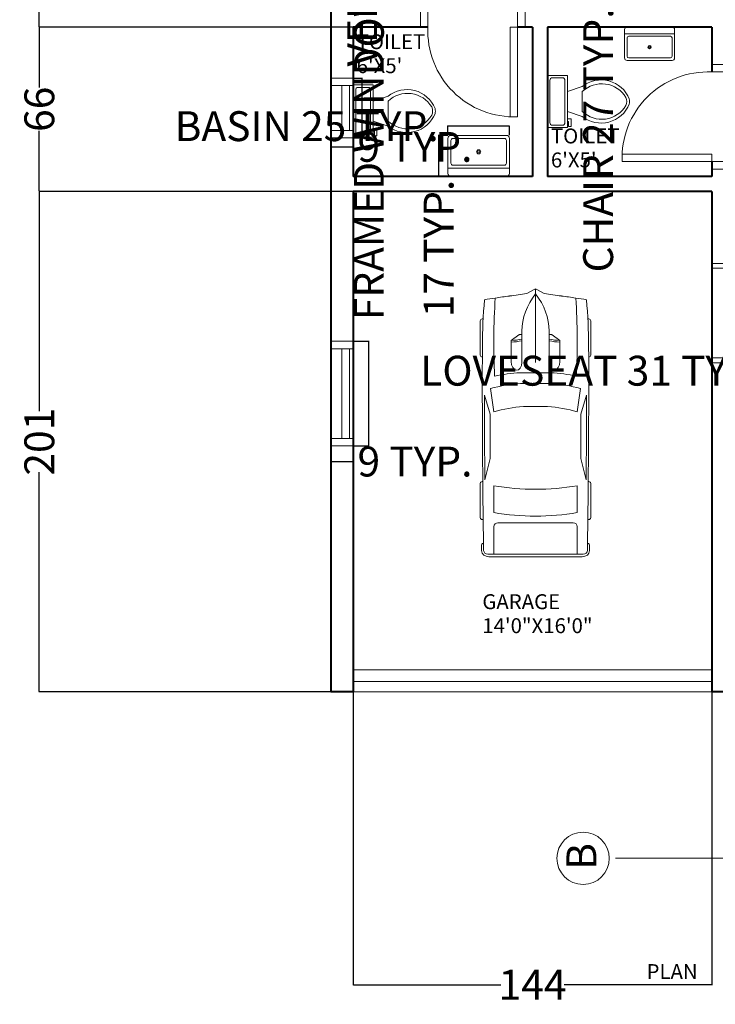
# Model space of a CAD drawing. Units: inches. Extents: x -101 to 786, y 26 to 880.
# Tile 1 of 9: x -101 to 178, y 26 to 422. Entities that reach past the tile are written whole.
import ezdxf

# ---------------------------------------------------------------- set-up
doc = ezdxf.new("R2010")
doc.units = ezdxf.units.IN
doc.header["$MEASUREMENT"] = 0
for name, color, linetype, lineweight in [('A-ANNO-DIMS', 2, 'Continuous', 18), ('A-ANNO-SYMB', 2, 'Continuous', 18), ('A-ANNO-TEXT', 7, 'Continuous', 25), ('A-AREA-IDEN', 7, 'Continuous', 18), ('A-DOOR', 4, 'Continuous', 20), ('A-EQPM-VEHC', 9, 'Continuous', 13), ('A-FLOR-FIXT', 8, 'Continuous', 18), ('A-GLAZ', 4, 'Continuous', 18), ('A-WALL', 7, 'Continuous', 40)]:
    doc.layers.add(name, color=color, linetype=linetype, lineweight=lineweight)
doc.styles.get("Standard").update_dxf_attribs({"font": 'arial.ttf'})
doc.dimstyles.get("Standard").update_dxf_attribs({"dimtxt": 12, "dimasz": 0.18, "dimexe": 0.18, "dimexo": 0.0625, "dimgap": 0.09, "dimtad": 0, "dimdec": 1, "dimzin": 0, "dimdsep": 46, "dimlunit": 3, "dimtxsty": 'Standard', "dimcen": 0.09, "dimadec": 0, "dimazin": 0, "dimtfac": 1, "dimtdec": 1, "dimtofl": 0, "dimtmove": 0, "dimatfit": 3, "dimfxl": 1, "dimtolj": 1, "dimtzin": 0, "dimarcsym": 0})

# ---------------------------------------------------------------- blocks, each defined once
blk = doc.blocks.new('Sink-single - 30 in top')
blk.add_line((-15, -3.999996), (15, -3.999996))
for points in [[(-13.5, 0), (13.5, 0)], [(-15, -18.499996), (-15, -1.5)], [(15, -1.5), (15, -18.499996)], [(-13.5, -17.499996), (-13.5, -6.499996)], [(-12.5, -5.499996), (12.5, -5.499996)], [(13.5, -6.499996), (13.5, -17.499996)], [(12.5, -18.499996), (-12.5, -18.499996)], [(13.5, -19.999996), (-13.5, -19.999996)]]:
    blk.add_lwpolyline(points)
for radius in [1, 0.5]:
    blk.add_circle((0, -11.999996), radius)
for centre, radius, start, end in [((-13.5, -1.5), 1.5, 90, 180), ((13.5, -1.5), 1.5, 0, 90), ((-12.5, -6.499996), 1, 90, 180), ((12.5, -6.499996), 1, 0, 90), ((-13.5, -18.499996), 1.5, 180, 270), ((-12.5, -17.499996), 1, 180, 270), ((12.5, -17.499996), 1, 270, 0), ((13.5, -18.499996), 1.5, 270, 0)]:
    blk.add_arc(centre, radius, start, end)
blk = doc.blocks.new('Toilet - top')
for p, q in [((9.5, -6), (9.5, -2)), ((-10, -8.5), (-8, -8.5)), ((-10, -9.5), (-10, -8.5)), ((-7, -9.5), (-10, -9.5)), ((-8, -8.5), (-8, -8)), ((-7, -8), (-7, -9.5)), ((-4, -8), (-6, -14)), ((4, -8), (6, -14)), ((4, -14), (-4, -14))]:
    blk.add_line(p, q)
blk.add_lwpolyline([(10.5, -8), (10.5, 0), (-10.5, 0), (-10.5, -8)], close=True)
for points in [[(-9.5, -2), (-9.5, -6)], [(8.5, -1), (-8.5, -1)], [(-8.5, -7), (8.5, -7)]]:
    blk.add_lwpolyline(points)
for centre, radius, start, end in [((-8.62, -1.88), 0.884, 81.8699, 188.1301), ((8.62, -1.88), 0.884, 351.8699, 98.1301), ((-8.62, -6.12), 0.884, 171.8699, 278.1301), ((8.62, -6.12), 0.884, 261.8699, 8.1301), ((3.52, -21.58), 12.17, 141.4691, 247.9714), ((4.2, -21.82), 11.33, 136.3677, 238.9468), ((-3.52, -21.58), 12.17, 292.0284, 38.5307), ((-4.2, -21.82), 11.33, 301.053, 43.6321), ((0, -27.88), 4, 245.7318, 294.2682), ((0, -29), 4, 254.8605, 285.1395)]:
    blk.add_arc(centre, radius, start, end)
blk = doc.blocks.new('*U14')
for p, q in [((21.1, 37.41), (21.1, 36.83)), ((46.55, 38.89), (22.35, 38.89)), ((47.8, 37.39), (47.8, 37.41)), ((87.99, 31.87), (74.76, 35.92)), ((134.31, 35.6), (119.29, 31.78)), ((135.45, 37.07), (135.45, 37.41)), ((136.7, 38.89), (160.9, 38.89)), ((162.15, 37.41), (162.15, 36.77)), ((70.03, 31.54), (86.41, 29.35)), ((138.42, 29.35), (157.25, 29.35)), ((186.47, 29.35), (167.01, 29.35)), ((186.47, -33.5), (186.47, 33.5)), ((188.4, -32.76), (188.4, 32.76)), ((164.52, 26.39), (164.52, -26.39)), ((32.27, 11.63), (36.13, 17.17)), ((36.13, 17.17), (50.94, 17.17)), ((29.77, 9.51), (51.68, 9.51)), ((32.12, 9.51), (32.12, 11.15)), ((58.92, -10.77), (58.92, 10.77)), ((66.55, -10.53), (66.55, 10.53)), ((82.74, 8.5), (82.74, -8.5)), ((186.47, -10.53), (186.47, 10.53)), ((3.27, 6.13), (0.1, 0.41)), ((0, 0), (51.68, 0)), ((0.1, -0.41), (3.27, -6.13)), ((29.77, -9.51), (51.68, -9.51)), ((32.12, -9.51), (32.12, -11.15)), ((32.27, -11.63), (36.13, -17.17)), ((36.13, -17.17), (50.94, -17.17)), ((86.41, -29.35), (70.03, -31.54)), ((87.99, -31.87), (74.76, -35.92)), ((134.31, -35.6), (119.29, -31.78)), ((157.25, -29.35), (138.42, -29.35)), ((167.01, -29.35), (186.47, -29.35)), ((21.1, -37.41), (21.1, -36.83)), ((46.55, -38.89), (22.35, -38.89)), ((47.8, -37.39), (47.8, -37.41)), ((135.45, -37.07), (135.45, -37.41)), ((136.7, -38.89), (160.9, -38.89)), ((162.15, -37.41), (162.15, -36.77))]:
    blk.add_line(p, q)
for centre, major_axis, ratio, start_param, end_param in [((266.03, -27.52), (0, 313.31), 0.842304, 1.367076, 1.39176), ((41.19, -490.86), (0, 528.23), 0.842304, 0.00281, 0.075598), ((22.35, 37.41), (0, -1.48), 0.842304, 3.141593, 4.712389), ((64.48, -10555.62), (0, 10593.03), 0.842304, -0.013397, 0.002797), ((46.55, 37.41), (0, 1.48), 0.842304, -1.570796, 0), ((64.48, -10555.62), (0, -10591.55), 0.842304, 3.133765, 3.140441), ((136.7, 37.41), (0, -1.48), 0.842304, 3.141593, 4.712389), ((160.9, 37.41), (0, 1.48), 0.842304, -1.570796, 0), ((180.63, 35.84), (0, 2.22), 0.842304, -0.013017, 1.249894), ((64.48, -10556.36), (0, 10595.31), 0.842304, -0.013397, -0.013017), ((183.98, 33.5), (0, -2.96), 0.842304, 1.570796, 3.128196), ((183.98, 32.76), (0, -5.25), 0.842304, 1.570796, 3.128196), ((259.18, -27.52), (0, -305.3), 0.842304, 4.528606, 4.561838), ((37.47, -593.96), (0, -623.33), 0.842304, 3.096046, 3.200911), ((134.4, 5.39), (0, -89.78), 0.842304, 4.449482, 4.652344), ((135.29, 5.39), (0, 81.77), 0.842304, 1.245306, 1.50788), ((149.6, 2.8), (0, -79.58), 0.842304, 4.372215, 4.640744), ((95.79, -3666.35), (0, -3698.24), 0.842304, 3.134049, 3.144098), ((17.08, 0), (0, 147.02), 0.842304, 4.511394, 4.913384), ((35.91, 0), (0, 147.02), 0.842304, 4.511394, 4.913384), ((167.01, 26.39), (0, 2.96), 0.842304, 0, 1.570796), ((-204.49, 52.4), (0, -250.96), 0.842304, 1.385369, 1.434372), ((13.04, 17.01), (0, 27.42), 0.842304, 4.435146, 4.718221), ((14.2, 17.01), (0, 27.42), 0.842304, 4.435146, 4.718221), ((50.79, 13.34), (6.34, -0.36), 0.603834, -1.395552, 1.581315), ((29.77, -46.66), (0, 56.17), 0.842304, 0, 0.590319), ((32.75, 11.15), (0, 0.74), 0.842304, 0.879714, 1.570796), ((0.62, 0), (0, -0.74), 0.842304, 4.131459, 5.293319), ((-204.49, -52.4), (0, 250.96), 0.842304, -1.434372, -1.385369), ((29.77, 46.66), (0, 56.17), 0.842304, 2.551274, 3.141593), ((32.75, -11.15), (0, -0.74), 0.842304, 4.712389, 5.403472), ((13.04, -17.01), (0, -27.42), 0.842304, 1.564964, 1.848039), ((14.2, -17.01), (0, -27.42), 0.842304, 1.564964, 1.848039), ((134.4, -5.39), (0, -89.78), 0.842304, -1.510751, -1.307889), ((135.29, -5.39), (0, -81.77), 0.842304, -1.50788, -1.245306), ((149.6, -2.8), (0, -79.58), 0.842304, -1.499151, -1.230623), ((259.18, 27.52), (0, 305.3), 0.842304, 1.721348, 1.754579), ((167.01, -26.39), (0, -2.96), 0.842304, 4.712389, 6.283185), ((266.03, 27.52), (0, 313.31), 0.842304, 1.749832, 1.774517), ((37.47, 593.96), (0, -623.33), 0.842304, -0.059319, 0.045547), ((95.79, 3666.35), (0, -3698.24), 0.842304, -0.002505, 0.007544), ((183.98, -33.5), (0, 2.96), 0.842304, 3.15499, 4.712389), ((183.98, -32.76), (0, -5.25), 0.842304, 0.013397, 1.570796), ((41.19, 490.86), (0, -528.23), 0.842304, -0.075598, -0.00281), ((22.35, -37.41), (0, 1.48), 0.842304, 1.570796, 3.141593), ((64.48, 10555.62), (0, 10593.03), 0.842304, 3.138796, 3.15499), ((46.55, -37.41), (0, -1.48), 0.842304, 0, 1.570796), ((64.48, 10555.62), (0, -10591.55), 0.842304, 0.001152, 0.007828), ((136.7, -37.41), (0, -1.48), 0.842304, -1.570796, 0), ((160.9, -37.41), (0, 1.48), 0.842304, 3.141593, 4.712389), ((180.63, -35.84), (0, -2.22), 0.842304, -1.249894, 0.013017), ((64.48, 10556.36), (0, 10595.31), 0.842304, 3.15461, 3.15499)]:
    blk.add_ellipse(centre, major_axis=major_axis, ratio=ratio, start_param=start_param, end_param=end_param)
at = {"extrusion": (0, 0, -1)}
blk.add_ellipse((50.79, -13.34), major_axis=(6.34, 0.36), ratio=0.603834, start_param=-1.395552, end_param=1.581315, dxfattribs=at)
blk = doc.blocks.new('DOOR-SINGLE-36')
for p, q in [((-39, 0), (-39, -6)), ((-36, 0), (-36, -6)), ((0, 0), (0, -6)), ((3, 0), (3, -6))]:
    blk.add_line(p, q)
blk.add_lwpolyline([(0, 0), (-3, 0), (-3, 36), (0, 36)], close=True)
blk.add_arc((-1.5, 1.5), 34.53, 87.5104, 182.4896)
blk = doc.blocks.new('WIN-36-WALL9-FRAMED')
for p, q in [((0, 42), (9, 42)), ((0, 3), (0, 39)), ((0, 39), (9, 39)), ((4.5, 3), (4.5, 39)), ((7.5, 3), (7.5, 39)), ((9, 39), (9, 3)), ((9, 3), (0, 3)), ((9, 0), (0, 0))]:
    blk.add_line(p, q)
blk = doc.blocks.new('VENT-18-WALL9')
for p, q in [((9, 24), (0, 24)), ((9, 21), (0, 21)), ((4.5, 3), (4.5, 21)), ((7.5, 3), (7.5, 21)), ((0, 3), (9, 3)), ((0, 0), (9, 0))]:
    blk.add_line(p, q)
blk = doc.blocks.new('*D31')
at = {"layer": 'A-ANNO-DIMS', "color": 0, "lineweight": -2, "transparency": 16777216}
for p, q in [((134.84, 458.3), (130.68, 458.3)), ((130.86, 458.12), (130.86, 431.48)), ((134.84, 431.3), (130.68, 431.3)), ((130.86, 431.3), (130.86, 431.12))]:
    blk.add_line(p, q, dxfattribs=at)
at = {"layer": 'A-ANNO-DIMS', "color": 0, "transparency": 16777216}
for points in [[(130.83, 458.12), (130.89, 458.12), (130.86, 458.3)], [(130.83, 431.48), (130.89, 431.48), (130.86, 431.3)]]:
    blk.add_solid(points, dxfattribs=at)
at = {"layer": 'Defpoints', "color": 0, "transparency": 16777216}
for p in [(134.91, 458.3), (130.86, 431.3), (134.91, 431.3)]:
    blk.add_point(p, dxfattribs=at)
at = {"layer": 'A-ANNO-DIMS', "color": 0, "transparency": 16777216, "insert": (130.86, 373.49), "char_height": 12, "attachment_point": 5, "rotation": 90}
blk.add_mtext('\\A1;CHAIR 27 TYP.', dxfattribs=at)
blk = doc.blocks.new('*D41')
at = {"layer": 'A-ANNO-DIMS', "color": 0, "lineweight": -2, "transparency": 16777216}
for p, q in [((70.53, 379.02), (70.35, 379.02)), ((70.53, 375.37), (70.53, 379.2)), ((95.1, 379.02), (70.71, 379.02)), ((95.28, 375.37), (95.28, 379.2))]:
    blk.add_line(p, q, dxfattribs=at)
at = {"layer": 'A-ANNO-DIMS', "color": 0, "transparency": 16777216}
for points in [[(70.71, 379.05), (70.71, 378.99), (70.53, 379.02)], [(95.1, 379.05), (95.1, 378.99), (95.28, 379.02)]]:
    blk.add_solid(points, dxfattribs=at)
at = {"layer": 'Defpoints', "color": 0, "transparency": 16777216}
for p in [(70.53, 379.02), (70.53, 375.3), (95.28, 375.3)]:
    blk.add_point(p, dxfattribs=at)
at = {"layer": 'A-ANNO-DIMS', "color": 0, "transparency": 16777216, "insert": (13.83, 379.02), "char_height": 12, "attachment_point": 5}
blk.add_mtext('\\A1;BASIN 25 TYP.', dxfattribs=at)
blk = doc.blocks.new('*D42')
at = {"layer": 'A-ANNO-DIMS', "color": 0, "lineweight": -2, "transparency": 16777216}
for p, q in [((70.46, 375.3), (66.63, 375.3)), ((66.81, 375.12), (66.81, 358.98)), ((70.46, 358.8), (66.63, 358.8)), ((66.81, 358.8), (66.81, 358.62))]:
    blk.add_line(p, q, dxfattribs=at)
at = {"layer": 'A-ANNO-DIMS', "color": 0, "transparency": 16777216}
for points in [[(66.78, 375.12), (66.84, 375.12), (66.81, 375.3)], [(66.78, 358.98), (66.84, 358.98), (66.81, 358.8)]]:
    blk.add_solid(points, dxfattribs=at)
at = {"layer": 'Defpoints', "color": 0, "transparency": 16777216}
for p in [(70.53, 375.3), (66.81, 358.8), (70.53, 358.8)]:
    blk.add_point(p, dxfattribs=at)
at = {"layer": 'A-ANNO-DIMS', "color": 0, "transparency": 16777216, "insert": (66.81, 329.89), "char_height": 12, "attachment_point": 5, "rotation": 90}
blk.add_mtext('\\A1;17 TYP.', dxfattribs=at)
blk = doc.blocks.new('*D51')
at = {"layer": 'A-ANNO-DIMS', "color": 0, "lineweight": -2, "transparency": 16777216}
for p, q in [((38.81, 292.61), (38.81, 292.79)), ((32.57, 292.61), (38.99, 292.61)), ((38.81, 250.79), (38.81, 292.43)), ((32.57, 250.61), (38.99, 250.61))]:
    blk.add_line(p, q, dxfattribs=at)
at = {"layer": 'A-ANNO-DIMS', "color": 0, "transparency": 16777216}
for points in [[(38.78, 292.43), (38.84, 292.43), (38.81, 292.61)], [(38.78, 250.79), (38.84, 250.79), (38.81, 250.61)]]:
    blk.add_solid(points, dxfattribs=at)
at = {"layer": 'Defpoints', "color": 0, "transparency": 16777216}
for p in [(32.51, 292.61), (38.81, 292.61), (32.51, 250.61)]:
    blk.add_point(p, dxfattribs=at)
at = {"layer": 'A-ANNO-DIMS', "color": 0, "transparency": 16777216, "insert": (38.81, 398.57), "char_height": 12, "attachment_point": 5, "rotation": 90}
blk.add_mtext('\\A1;FRAMED WINDOW 42 TYP.', dxfattribs=at)
blk = doc.blocks.new('*D52')
at = {"layer": 'A-ANNO-DIMS', "color": 0, "lineweight": -2, "transparency": 16777216}
for p, q in [((23.51, 250.55), (23.51, 244.13)), ((32.51, 250.55), (32.51, 244.13)), ((23.69, 244.31), (32.33, 244.31)), ((32.51, 244.31), (32.69, 244.31))]:
    blk.add_line(p, q, dxfattribs=at)
at = {"layer": 'A-ANNO-DIMS', "color": 0, "transparency": 16777216}
for points in [[(23.69, 244.34), (23.69, 244.28), (23.51, 244.31)], [(32.33, 244.34), (32.33, 244.28), (32.51, 244.31)]]:
    blk.add_solid(points, dxfattribs=at)
at = {"layer": 'Defpoints', "color": 0, "transparency": 16777216}
for p in [(23.51, 250.61), (32.51, 250.61), (32.51, 244.31)]:
    blk.add_point(p, dxfattribs=at)
at = {"layer": 'A-ANNO-DIMS', "color": 0, "transparency": 16777216, "insert": (57.32, 244.31), "char_height": 12, "attachment_point": 5}
blk.add_mtext('\\A1;9 TYP.', dxfattribs=at)
blk = doc.blocks.new('*D55')
at = {"layer": 'A-ANNO-DIMS', "color": 0, "lineweight": -2, "transparency": 16777216}
for p, q in [((204.29, 276.16), (204.29, 280.97)), ((235.59, 276.16), (235.59, 280.97)), ((204.29, 280.79), (204.11, 280.79)), ((235.41, 280.79), (204.47, 280.79))]:
    blk.add_line(p, q, dxfattribs=at)
at = {"layer": 'A-ANNO-DIMS', "color": 0, "transparency": 16777216}
for points in [[(204.47, 280.82), (204.47, 280.76), (204.29, 280.79)], [(235.41, 280.82), (235.41, 280.76), (235.59, 280.79)]]:
    blk.add_solid(points, dxfattribs=at)
at = {"layer": 'Defpoints', "color": 0, "transparency": 16777216}
for p in [(204.29, 280.79), (204.29, 276.1), (235.59, 276.1)]:
    blk.add_point(p, dxfattribs=at)
at = {"layer": 'A-ANNO-DIMS', "color": 0, "transparency": 16777216, "insert": (128.5, 280.79), "char_height": 12, "attachment_point": 5}
blk.add_mtext('\\A1;LOVESEAT 31 TYP.', dxfattribs=at)
blk = doc.blocks.new('*D59')
at = {"layer": 'A-ANNO-DIMS', "color": 0, "lineweight": -2, "transparency": 16777216}
for p, q in [((32.57, 398.32), (36.29, 398.32)), ((36.11, 398.32), (36.11, 398.5)), ((36.11, 374.5), (36.11, 398.14)), ((32.57, 374.32), (36.29, 374.32))]:
    blk.add_line(p, q, dxfattribs=at)
at = {"layer": 'A-ANNO-DIMS', "color": 0, "transparency": 16777216}
for points in [[(36.08, 398.14), (36.14, 398.14), (36.11, 398.32)], [(36.08, 374.5), (36.14, 374.5), (36.11, 374.32)]]:
    blk.add_solid(points, dxfattribs=at)
at = {"layer": 'Defpoints', "color": 0, "transparency": 16777216}
for p in [(32.51, 398.32), (36.11, 398.32), (32.51, 374.32)]:
    blk.add_point(p, dxfattribs=at)
at = {"layer": 'A-ANNO-DIMS', "color": 0, "transparency": 16777216, "insert": (36.11, 452.79), "char_height": 12, "attachment_point": 5, "rotation": 90}
blk.add_mtext('\\A1;VENT 24 TYP.', dxfattribs=at)
blk = doc.blocks.new('*D60')
at = {"layer": 'A-ANNO-DIMS', "color": 0, "lineweight": -2, "transparency": 16777216}
for p, q in [((23.51, 374.26), (23.51, 370.54)), ((32.51, 374.26), (32.51, 370.54)), ((23.69, 370.72), (32.33, 370.72)), ((32.51, 370.72), (32.69, 370.72))]:
    blk.add_line(p, q, dxfattribs=at)
at = {"layer": 'A-ANNO-DIMS', "color": 0, "transparency": 16777216}
for points in [[(23.69, 370.75), (23.69, 370.69), (23.51, 370.72)], [(32.33, 370.75), (32.33, 370.69), (32.51, 370.72)]]:
    blk.add_solid(points, dxfattribs=at)
at = {"layer": 'Defpoints', "color": 0, "transparency": 16777216}
for p in [(23.51, 374.32), (32.51, 374.32), (32.51, 370.72)]:
    blk.add_point(p, dxfattribs=at)
at = {"layer": 'A-ANNO-DIMS', "color": 0, "transparency": 16777216, "insert": (57.32, 370.72), "char_height": 12, "attachment_point": 5}
blk.add_mtext('\\A1;9 TYP.', dxfattribs=at)
blk = doc.blocks.new('*D73')
at = {"layer": 'A-ANNO-DIMS', "color": 0, "lineweight": -2, "transparency": 16777216}
for p, q in [((208.06, 316.53), (202.63, 316.53)), ((202.81, 316.35), (202.81, 281.31)), ((208.06, 281.13), (202.63, 281.13)), ((202.81, 281.13), (202.81, 280.95))]:
    blk.add_line(p, q, dxfattribs=at)
at = {"layer": 'A-ANNO-DIMS', "color": 0, "transparency": 16777216}
for points in [[(202.78, 316.35), (202.84, 316.35), (202.81, 316.53)], [(202.78, 281.31), (202.84, 281.31), (202.81, 281.13)]]:
    blk.add_solid(points, dxfattribs=at)
at = {"layer": 'Defpoints', "color": 0, "transparency": 16777216}
for p in [(208.12, 316.53), (202.81, 281.13), (208.12, 281.13)]:
    blk.add_point(p, dxfattribs=at)
at = {"layer": 'A-ANNO-DIMS', "color": 0, "transparency": 16777216, "insert": (202.81, 207.08), "char_height": 12, "attachment_point": 5, "rotation": 90}
blk.add_mtext('\\A1;COFFEE TABLE 35', dxfattribs=at)
blk = doc.blocks.new('*D81')
at = {"layer": 'A-ANNO-DIMS', "color": 0, "lineweight": -2, "transparency": 16777216}
for p, q in [((32.44, 352.8), (-93.7, 352.8)), ((-93.52, 352.62), (-93.52, 264.59)), ((-93.52, 151.98), (-93.52, 240.01)), ((23.44, 151.8), (-93.7, 151.8))]:
    blk.add_line(p, q, dxfattribs=at)
at = {"layer": 'A-ANNO-DIMS', "color": 0, "transparency": 16777216}
for points in [[(-93.55, 352.62), (-93.49, 352.62), (-93.52, 352.8)], [(-93.55, 151.98), (-93.49, 151.98), (-93.52, 151.8)]]:
    blk.add_solid(points, dxfattribs=at)
at = {"layer": 'Defpoints', "color": 0, "transparency": 16777216}
for p in [(-93.52, 352.8), (32.51, 352.8), (23.51, 151.8)]:
    blk.add_point(p, dxfattribs=at)
at = {"layer": 'A-ANNO-DIMS', "color": 0, "transparency": 16777216, "insert": (-93.52, 252.3), "char_height": 12, "attachment_point": 5, "rotation": 90}
blk.add_mtext('\\A1;201', dxfattribs=at)
blk = doc.blocks.new('*D82')
at = {"layer": 'A-ANNO-DIMS', "color": 0, "lineweight": -2, "transparency": 16777216}
for p, q in [((32.44, 418.8), (-93.7, 418.8)), ((-93.52, 418.62), (-93.52, 394.52)), ((-93.52, 352.98), (-93.52, 377.09)), ((32.44, 352.8), (-93.7, 352.8))]:
    blk.add_line(p, q, dxfattribs=at)
at = {"layer": 'A-ANNO-DIMS', "color": 0, "transparency": 16777216}
for points in [[(-93.55, 418.62), (-93.49, 418.62), (-93.52, 418.8)], [(-93.55, 352.98), (-93.49, 352.98), (-93.52, 352.8)]]:
    blk.add_solid(points, dxfattribs=at)
at = {"layer": 'Defpoints', "color": 0, "transparency": 16777216}
for p in [(-93.52, 418.8), (32.51, 418.8), (32.51, 352.8)]:
    blk.add_point(p, dxfattribs=at)
at = {"layer": 'A-ANNO-DIMS', "color": 0, "transparency": 16777216, "insert": (-93.52, 385.8), "char_height": 12, "attachment_point": 5, "rotation": 90}
blk.add_mtext('\\A1;66', dxfattribs=at)
blk = doc.blocks.new('*D83')
at = {"layer": 'A-ANNO-DIMS', "color": 0, "lineweight": -2, "transparency": 16777216}
for p, q in [((32.44, 556.8), (-93.7, 556.8)), ((-93.52, 556.62), (-93.52, 500.6)), ((-93.52, 418.98), (-93.52, 475.01)), ((32.44, 418.8), (-93.7, 418.8))]:
    blk.add_line(p, q, dxfattribs=at)
at = {"layer": 'A-ANNO-DIMS', "color": 0, "transparency": 16777216}
for points in [[(-93.55, 556.62), (-93.49, 556.62), (-93.52, 556.8)], [(-93.55, 418.98), (-93.49, 418.98), (-93.52, 418.8)]]:
    blk.add_solid(points, dxfattribs=at)
at = {"layer": 'Defpoints', "color": 0, "transparency": 16777216}
for p in [(-93.52, 556.8), (32.51, 556.8), (32.51, 418.8)]:
    blk.add_point(p, dxfattribs=at)
at = {"layer": 'A-ANNO-DIMS', "color": 0, "transparency": 16777216, "insert": (-93.52, 487.8), "char_height": 12, "attachment_point": 5, "rotation": 90}
blk.add_mtext('\\A1;138', dxfattribs=at)
blk = doc.blocks.new('*D86')
at = {"layer": 'A-ANNO-DIMS', "color": 0, "lineweight": -2, "transparency": 16777216}
for p, q in [((32.51, 151.74), (32.51, 33.98)), ((176.51, 151.74), (176.51, 33.98)), ((32.69, 34.16), (91.75, 34.16)), ((176.33, 34.16), (117.26, 34.16))]:
    blk.add_line(p, q, dxfattribs=at)
at = {"layer": 'A-ANNO-DIMS', "color": 0, "transparency": 16777216}
for points in [[(32.69, 34.19), (32.69, 34.13), (32.51, 34.16)], [(176.33, 34.19), (176.33, 34.13), (176.51, 34.16)]]:
    blk.add_solid(points, dxfattribs=at)
at = {"layer": 'Defpoints', "color": 0, "transparency": 16777216}
for p in [(32.51, 151.8), (176.51, 151.8), (176.51, 34.16)]:
    blk.add_point(p, dxfattribs=at)
at = {"layer": 'A-ANNO-DIMS', "color": 0, "transparency": 16777216, "insert": (104.51, 34.16), "char_height": 12, "attachment_point": 5}
blk.add_mtext('\\A1;144', dxfattribs=at)

msp = doc.modelspace()

# ---------------------------------------------------------------- linework, layer by layer
at = {"layer": 'A-ANNO-SYMB'}
msp.add_line((183.8117, 84.9238), (137.8117, 84.9238), dxfattribs=at)
msp.add_circle((124.8117, 84.9238), 10.5119, dxfattribs=at)
at = {"layer": 'A-DOOR'}
for p, q in [((32.5071, 160.6465), (176.5071, 160.6465)), ((32.5071, 156.0176), (176.5071, 156.0176)), ((32.5071, 151.8033), (176.5071, 151.8033))]:
    msp.add_line(p, q, dxfattribs=at)
at = {"layer": 'A-GLAZ'}
for p, q in [((182.5071, 323.9238), (176.5071, 323.9238)), ((182.5071, 321.9238), (176.5071, 321.9238)), ((176.5071, 285.9238), (182.5071, 285.9238)), ((176.5071, 283.9238), (182.5071, 283.9238))]:
    msp.add_line(p, q, dxfattribs=at)
at = {"layer": 'A-WALL'}
for p, q in [((32.5071, 418.8033), (32.5071, 358.8033)), ((62.5071, 418.8033), (32.5071, 418.8033)), ((104.5071, 418.8033), (98.5071, 418.8033)), ((104.5071, 418.8033), (104.5071, 358.8033)), ((176.5071, 418.8033), (110.5071, 418.8033)), ((110.5071, 418.8033), (110.5071, 358.8033)), ((176.5071, 418.8033), (176.5071, 400.8033)), ((176.5071, 364.8033), (176.5071, 358.8033)), ((104.5071, 358.8033), (32.5071, 358.8033)), ((176.5071, 358.8033), (110.5071, 358.8033)), ((176.5071, 352.8033), (32.5071, 352.8033)), ((32.5071, 352.8033), (32.5071, 151.8033)), ((176.5071, 352.8033), (176.5071, 151.8033)), ((32.5071, 151.8033), (23.5071, 151.8033)), ((182.5071, 151.8033), (176.5071, 151.8033))]:
    msp.add_line(p, q, dxfattribs=at)
msp.add_lwpolyline([(323.5071, 151.8033), (323.5071, 781.8033), (23.5071, 781.8033), (23.5071, 151.8033)], dxfattribs=at)

# ---------------------------------------------------------------- block references
at = {"layer": 'A-DOOR', "extrusion": (0, 0, -1), "zscale": -1}
for p, rotation in [((-98.5071, 418.8033), 180), ((-176.5071, 364.8033), 270.0000000000001)]:
    msp.add_blockref('DOOR-SINGLE-36', p, dxfattribs=dict(at, rotation=rotation))
at = {"layer": 'A-EQPM-VEHC', "xscale": 0.5710258329299738, "yscale": 0.5710258329299738, "zscale": 0.5710258329299738, "rotation": 269.9999999999969}
msp.add_blockref('*U14', (105.7191, 313.6193), dxfattribs=at)
at = {"layer": 'A-FLOR-FIXT', "xscale": 0.669901374782416, "yscale": 0.669901374782416, "zscale": 0.669901374782416}
msp.add_blockref('Sink-single - 30 in top', (151.4983, 418.8033), dxfattribs=at)
at = {"layer": 'A-FLOR-FIXT', "rotation": 90}
for p in [(32.5071, 385.0802), (110.5071, 388.9281)]:
    msp.add_blockref('Toilet - top', p, dxfattribs=at)
at = {"layer": 'A-FLOR-FIXT', "xscale": 0.8250378517028346, "yscale": 0.8250378517028346, "zscale": 0.8250378517028346, "rotation": 180}
msp.add_blockref('Sink-single - 30 in top', (82.9007, 358.8033), dxfattribs=at)
at = {"layer": 'A-GLAZ'}
for name, p in [('VENT-18-WALL9', (23.507, 374.32)), ('WIN-36-WALL9-FRAMED', (23.507, 250.6106))]:
    msp.add_blockref(name, p, dxfattribs=at)

# ---------------------------------------------------------------- texts
at = {"layer": 'A-ANNO-SYMB'}
msp.add_text('B', height=12, rotation=90, dxfattribs=at).set_placement((130.1391, 80.317))
at = {"layer": 'A-ANNO-TEXT'}
msp.add_text('PLAN', height=6, dxfattribs=at).set_placement((150.3117, 36.4238))
at = {"layer": 'A-AREA-IDEN'}
for s, p in [('TOILET', (33.9055, 409.9551)), ("6'X5'", (33.9055, 400.3166)), ('TOILET', (111.9078, 372.0875)), ("6'X5'", (111.9078, 362.449)), ('GARAGE', (84.3595, 185.0101)), ('14\'0"X16\'0"', (84.3595, 175.3717))]:
    msp.add_text(s, height=6, dxfattribs=at).set_placement(p)

# ---------------------------------------------------------------- dimensions: what is measured, and where the dimension line sits
at = {"layer": 'A-ANNO-DIMS'}
for base, p1, p2, picture, middle in [((-93.5225, 556.8033), (32.5071, 418.8033), (32.5071, 556.8033), '*D83', (-93.5225, 487.8033)), ((-93.5225, 418.8033), (32.5071, 352.8033), (32.5071, 418.8033), '*D82', (-93.5225, 385.8033)), ((-93.5225, 352.8033), (23.5071, 151.8033), (32.5071, 352.8033), '*D81', (-93.5225, 252.3033))]:
    dim = msp.add_linear_dim(base=base, p1=p1, p2=p2, angle=90, dimstyle='Standard', override={"dimdec": 0, "dimlfac": 1, "dimrnd": 0, "dimzin": 0, "dimdsep": 46, "dimlunit": 2}, dxfattribs=at)
    dim.commit()
    dim.dimension.update_dxf_attribs({"geometry": picture, "text_midpoint": middle})
for base, p1, p2, angle, text, picture, middle in [((36.1071, 398.3203), (32.5071, 374.3203), (32.5071, 398.3203), 90, 'VENT <> TYP.', '*D59', (36.1071, 452.7908)), ((38.8071, 292.6111), (32.5071, 250.6111), (32.5071, 292.6111), 90, 'FRAMED WINDOW <> TYP.', '*D51', (38.8071, 398.5728)), ((130.8566, 431.3033), (134.9066, 458.3033), (134.9066, 431.3033), 270.000001, 'CHAIR <> TYP.', '*D31', (130.8566, 373.489)), ((70.5252, 379.0167), (95.2763, 375.3041), (70.5252, 375.3041), 180, 'BASIN <> TYP.', '*D41', (13.8323, 379.0167)), ((66.8125, 358.8033), (70.5252, 375.3041), (70.5252, 358.8033), 270, '<> TYP.', '*D42', (66.8125, 329.8921)), ((202.8101, 281.1264), (208.1204, 316.5288), (208.1204, 281.1264), 270, 'COFFEE TABLE <>', '*D73', (202.8101, 207.0801)), ((204.2926, 280.791), (235.5878, 276.0967), (204.2926, 276.0967), 180, 'LOVESEAT <> TYP.', '*D55', (128.4988, 280.791))]:
    dim = msp.add_linear_dim(base=base, p1=p1, p2=p2, angle=angle, text=text, dimstyle='Standard', override={"dimdec": 0, "dimlfac": 1, "dimrnd": 0, "dimzin": 0, "dimdsep": 46, "dimlunit": 2}, dxfattribs=at)
    dim.commit()
    dim.dimension.update_dxf_attribs({"geometry": picture, "text_midpoint": middle})
for base, p1, p2, picture, middle in [((32.5071, 370.7203), (23.5071, 374.3203), (32.5071, 374.3203), '*D60', (57.3214, 370.7203)), ((32.5071, 244.3111), (23.5071, 250.6111), (32.5071, 250.6111), '*D52', (57.3214, 244.3111))]:
    dim = msp.add_linear_dim(base=base, p1=p1, p2=p2, text='<> TYP.', dimstyle='Standard', override={"dimdec": 0, "dimlfac": 1, "dimrnd": 0, "dimzin": 0, "dimdsep": 46, "dimlunit": 2}, dxfattribs=at)
    dim.commit()
    dim.dimension.update_dxf_attribs({"geometry": picture, "text_midpoint": middle})
dim = msp.add_linear_dim(base=(176.5071, 34.1619), p1=(32.5071, 151.8033), p2=(176.5071, 151.8033), dimstyle='Standard', override={"dimdec": 0, "dimlfac": 1, "dimrnd": 0, "dimzin": 0, "dimdsep": 46, "dimlunit": 2}, dxfattribs=at)
dim.commit()
dim.dimension.update_dxf_attribs({"geometry": '*D86', "text_midpoint": (104.5071, 34.1619)})

doc.saveas('drawing.dxf')
